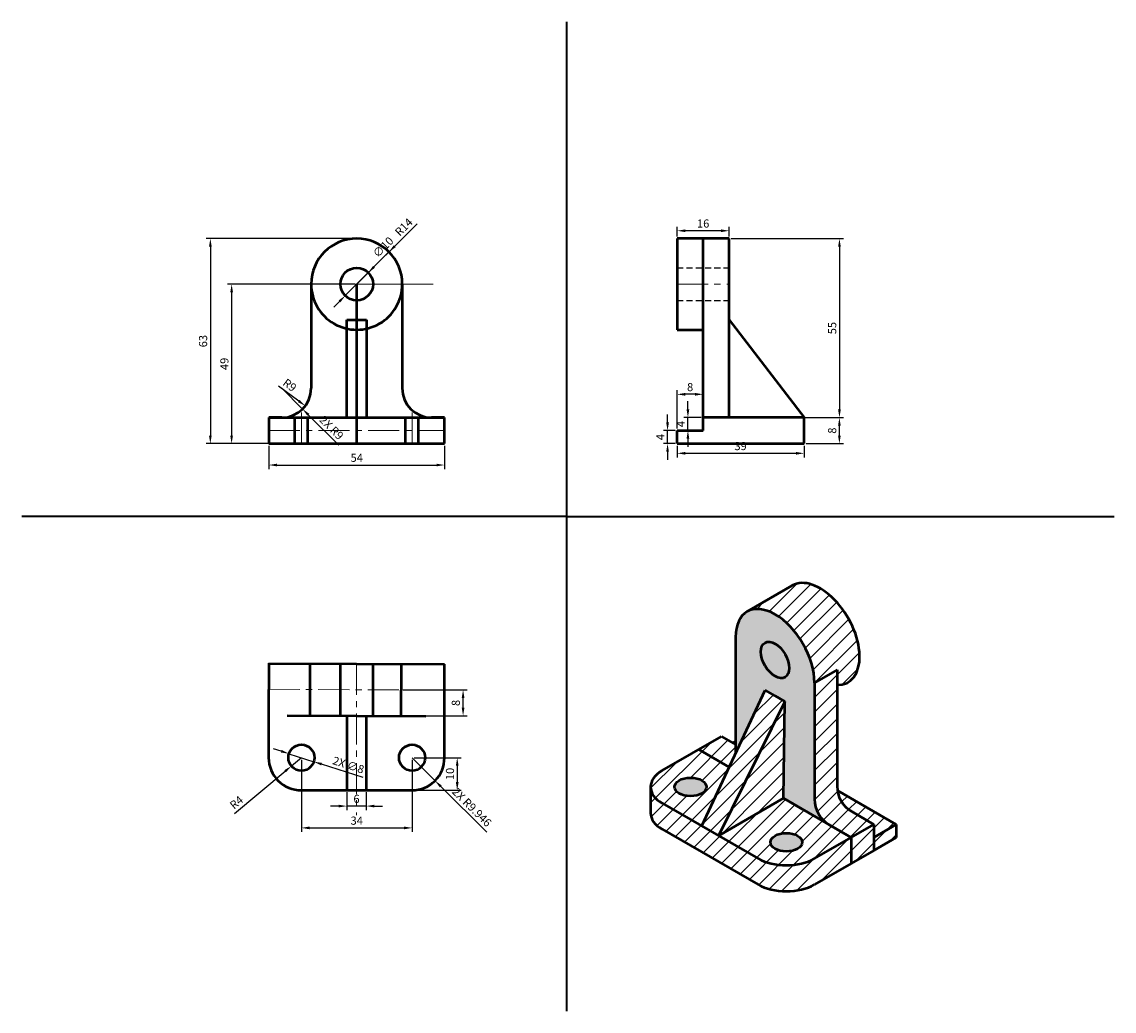
# Model space of a CAD drawing. Units: millimetres. Extents: x 2643 to 3341, y 1496 to 1804.
# Tile 2 of 2: x 3006 to 3341, y 1496 to 1800. Entities that reach past the tile are written whole.
import ezdxf

# ---------------------------------------------------------------- set-up
doc = ezdxf.new("R2010")
doc.units = ezdxf.units.MM
doc.linetypes.add('CENTER', pattern=[50.800000000000004, 31.75, -6.349999999999999, 6.349999999999999, -6.349999999999999])
doc.linetypes.add('HIDDEN', pattern=[9.524999999999999, 6.349999999999999, -3.174999999999999])
for name, color, linetype, lineweight in [('M-CNTR', 1, 'CENTER', 18), ('M-DIMS', 2, 'Continuous', 25), ('M-HATC', 252, 'Continuous', 18), ('M-HIDN', 4, 'HIDDEN', 25), ('M-OUTL', 7, 'Continuous', 50), ('M-TTLB', 8, 'Continuous', 35)]:
    doc.layers.add(name, color=color, linetype=linetype, lineweight=lineweight)
doc.styles.get("Standard").update_dxf_attribs({"font": 'arial.ttf'})
doc.dimstyles.new('ISO-25', dxfattribs={"dimtxt": 2.5, "dimasz": 2.5, "dimexe": 1.25, "dimexo": 0.625, "dimtad": 1, "dimtxsty": 'Standard', "dimcen": 2.5, "dimadec": 0, "dimazin": 0, "dimtfac": 1, "dimtmove": 0, "dimatfit": 3, "dimfxl": 1, "dimarcsym": 0})

# ---------------------------------------------------------------- blocks, each defined once
blk = doc.blocks.new('*D17')
at = {"layer": 'Defpoints', "color": 0, "transparency": 16777216}
for p in [(3081.566068859823, 1670.192632405238), (3135.566068859823, 1670.192632405237), (3135.566068859823, 1663.625483278832)]:
    blk.add_point(p, dxfattribs=at)
at = {"layer": 'M-DIMS', "color": 0, "lineweight": -2, "transparency": 16777216}
for p, q in [((3081.566068859823, 1669.567632405238), (3081.566068859823, 1662.375483278832)), ((3135.566068859823, 1669.567632405238), (3135.566068859823, 1662.375483278832)), ((3084.066068859823, 1663.625483278832), (3133.066068859823, 1663.625483278832))]:
    blk.add_line(p, q, dxfattribs=at)
at = {"layer": 'M-DIMS', "color": 0, "transparency": 16777216}
for points in [[(3084.066068859823, 1664.042149945499), (3084.066068859823, 1663.208816612165), (3081.566068859823, 1663.625483278832)], [(3133.066068859823, 1664.042149945499), (3133.066068859823, 1663.208816612165), (3135.566068859823, 1663.625483278832)]]:
    blk.add_solid(points, dxfattribs=at)
at = {"layer": 'M-DIMS', "color": 0, "transparency": 16777216, "insert": (3108.566068859823, 1665.521799786336), "char_height": 2.5, "attachment_point": 5}
blk.add_mtext('54', dxfattribs=at)
blk = doc.blocks.new('*D18')
at = {"layer": 'Defpoints', "color": 0, "transparency": 16777216}
for p in [(3085.566068859823, 1687.192632405238), (3092.76814055005, 1681.795395763327)]:
    blk.add_point(p, dxfattribs=at)
at = {"layer": 'M-DIMS', "color": 0, "lineweight": -2, "transparency": 16777216}
blk.add_line((3084.536577635948, 1687.964133716945), (3090.767565080541, 1683.294628163858), dxfattribs=at)
at = {"layer": 'M-DIMS', "color": 0, "transparency": 16777216}
blk.add_solid([(3091.017437147297, 1683.628057408776), (3090.517693013787, 1682.961198918941), (3092.76814055005, 1681.795395763327)], dxfattribs=at)
at = {"layer": 'M-DIMS', "color": 0, "transparency": 16777216, "insert": (3087.792059289652, 1687.900580802674), "char_height": 2.5, "attachment_point": 5, "rotation": 323.15208929564767}
blk.add_mtext('R9', dxfattribs=at)
blk = doc.blocks.new('*D19')
at = {"layer": 'Defpoints', "color": 0, "transparency": 16777216}
for p in [(3108.566068859825, 1719.192632405238), (3070.137380430236, 1670.192632405238), (3108.566068859825, 1670.192632405238)]:
    blk.add_point(p, dxfattribs=at)
at = {"layer": 'M-DIMS', "color": 0, "lineweight": -2, "transparency": 16777216}
for p, q in [((3107.941068859825, 1719.192632405238), (3068.887380430236, 1719.192632405238)), ((3070.137380430236, 1716.692632405238), (3070.137380430236, 1672.692632405238)), ((3107.941068859825, 1670.192632405238), (3068.887380430236, 1670.192632405238))]:
    blk.add_line(p, q, dxfattribs=at)
at = {"layer": 'M-DIMS', "color": 0, "transparency": 16777216}
for points in [[(3069.720713763569, 1716.692632405238), (3070.554047096902, 1716.692632405238), (3070.137380430236, 1719.192632405238)], [(3069.720713763569, 1672.692632405238), (3070.554047096902, 1672.692632405238), (3070.137380430236, 1670.192632405238)]]:
    blk.add_solid(points, dxfattribs=at)
at = {"layer": 'M-DIMS', "color": 0, "transparency": 16777216, "insert": (3068.235947960932, 1694.692632405236), "char_height": 2.5, "attachment_point": 5, "rotation": 90}
blk.add_mtext('49', dxfattribs=at)
blk = doc.blocks.new('*D20')
at = {"layer": 'Defpoints', "color": 0, "transparency": 16777216}
for p in [(3108.566068859825, 1733.192632405238), (3063.600548809042, 1670.192632405239), (3108.566068859825, 1670.192632405239)]:
    blk.add_point(p, dxfattribs=at)
at = {"layer": 'M-DIMS', "color": 0, "lineweight": -2, "transparency": 16777216}
for p, q in [((3107.941068859825, 1733.192632405238), (3062.350548809043, 1733.192632405238)), ((3063.600548809042, 1730.692632405238), (3063.600548809042, 1672.692632405239)), ((3107.941068859825, 1670.192632405239), (3062.350548809043, 1670.192632405239))]:
    blk.add_line(p, q, dxfattribs=at)
at = {"layer": 'M-DIMS', "color": 0, "transparency": 16777216}
for points in [[(3063.183882142376, 1730.692632405238), (3064.017215475709, 1730.692632405238), (3063.600548809042, 1733.192632405238)], [(3063.183882142376, 1672.692632405239), (3064.017215475709, 1672.692632405239), (3063.600548809042, 1670.192632405239)]]:
    blk.add_solid(points, dxfattribs=at)
at = {"layer": 'M-DIMS', "color": 0, "transparency": 16777216, "insert": (3061.698263679438, 1701.692632405237), "char_height": 2.5, "attachment_point": 5, "rotation": 90}
blk.add_mtext('63', dxfattribs=at)
blk = doc.blocks.new('*D21')
at = {"layer": 'Defpoints', "color": 0, "transparency": 16777216}
for p in [(3091.566068859822, 1573.72030741397), (3088.49388517497, 1571.158728329402)]:
    blk.add_point(p, dxfattribs=at)
at = {"layer": 'M-DIMS', "color": 0, "lineweight": -2, "transparency": 16777216}
for p, q in [((3091.566068859822, 1573.72030741397), (3088.49388517497, 1571.158728329402)), ((3071.01828682517, 1556.587618065424), (3086.573770371936, 1569.557741401545))]:
    blk.add_line(p, q, dxfattribs=at)
at = {"layer": 'M-DIMS', "color": 0, "transparency": 16777216}
blk.add_solid([(3086.306939217294, 1569.877760535384), (3086.840601526579, 1569.237722267706), (3088.49388517497, 1571.158728329402)], dxfattribs=at)
at = {"layer": 'M-DIMS', "color": 0, "transparency": 16777216, "insert": (3071.841787712557, 1559.715511328002), "char_height": 2.5, "attachment_point": 5, "rotation": 39.821262890870386}
blk.add_mtext('R4', dxfattribs=at)
blk = doc.blocks.new('*D22')
at = {"layer": 'Defpoints', "color": 0, "transparency": 16777216}
for p in [(3091.566068859821, 1573.720307413966), (3125.566068859823, 1573.72030741397), (3125.566068859823, 1552.148762047337)]:
    blk.add_point(p, dxfattribs=at)
at = {"layer": 'M-DIMS', "color": 0, "lineweight": -2, "transparency": 16777216}
for p, q in [((3091.566068859821, 1573.095307413966), (3091.566068859821, 1550.898762047337)), ((3125.566068859823, 1573.09530741397), (3125.566068859823, 1550.898762047337)), ((3094.066068859821, 1552.148762047337), (3123.066068859823, 1552.148762047337))]:
    blk.add_line(p, q, dxfattribs=at)
at = {"layer": 'M-DIMS', "color": 0, "transparency": 16777216}
for points in [[(3094.066068859821, 1552.565428714004), (3094.066068859821, 1551.73209538067), (3091.566068859821, 1552.148762047337)], [(3123.066068859823, 1552.565428714004), (3123.066068859823, 1551.73209538067), (3125.566068859823, 1552.148762047337)]]:
    blk.add_solid(points, dxfattribs=at)
at = {"layer": 'M-DIMS', "color": 0, "transparency": 16777216, "insert": (3108.566068859822, 1554.051047176942), "char_height": 2.5, "attachment_point": 5}
blk.add_mtext('34', dxfattribs=at)
blk = doc.blocks.new('*D23')
at = {"layer": 'Defpoints', "color": 0, "transparency": 16777216}
for p in [(3105.493192340093, 1563.72030741397), (3111.493192340093, 1563.720307413971), (3105.493192340093, 1558.848600236895)]:
    blk.add_point(p, dxfattribs=at)
at = {"layer": 'M-DIMS', "color": 0, "lineweight": -2, "transparency": 16777216}
for p, q in [((3105.493192340093, 1563.095307413971), (3105.493192340093, 1557.598600236896)), ((3111.493192340093, 1563.095307413971), (3111.493192340093, 1557.598600236896)), ((3102.993192340093, 1558.848600236895), (3100.493192340093, 1558.848600236895)), ((3111.493192340093, 1558.848600236895), (3105.493192340093, 1558.848600236895)), ((3113.993192340093, 1558.848600236895), (3116.493192340093, 1558.848600236895))]:
    blk.add_line(p, q, dxfattribs=at)
at = {"layer": 'M-DIMS', "color": 0, "transparency": 16777216}
for points in [[(3102.993192340093, 1559.265266903562), (3102.993192340093, 1558.431933570229), (3105.493192340093, 1558.848600236895)], [(3113.993192340093, 1559.265266903562), (3113.993192340093, 1558.431933570229), (3111.493192340093, 1558.848600236895)]]:
    blk.add_solid(points, dxfattribs=at)
at = {"layer": 'M-DIMS', "color": 0, "transparency": 16777216, "insert": (3108.493192340093, 1560.7500327062), "char_height": 2.5, "attachment_point": 5}
blk.add_mtext('6', dxfattribs=at)
blk = doc.blocks.new('*D24')
at = {"layer": 'Defpoints', "color": 0, "transparency": 16777216}
for p in [(3125.566068859825, 1573.720307413971), (3125.593251720514, 1563.720344158577), (3139.428818305797, 1563.720344158577)]:
    blk.add_point(p, dxfattribs=at)
at = {"layer": 'M-DIMS', "color": 0, "lineweight": -2, "transparency": 16777216}
for p, q in [((3126.191068859825, 1573.720307413971), (3140.678818305797, 1573.720307413971)), ((3139.428818305797, 1571.220307413971), (3139.428818305797, 1566.220344158577)), ((3126.218251720513, 1563.720344158577), (3140.678818305797, 1563.720344158577))]:
    blk.add_line(p, q, dxfattribs=at)
at = {"layer": 'M-DIMS', "color": 0, "transparency": 16777216}
for points in [[(3139.012151639131, 1571.220307413971), (3139.845484972464, 1571.220307413971), (3139.428818305797, 1573.720307413971)], [(3139.012151639131, 1566.220344158577), (3139.845484972464, 1566.220344158577), (3139.428818305797, 1563.720344158577)]]:
    blk.add_solid(points, dxfattribs=at)
at = {"layer": 'M-DIMS', "color": 0, "transparency": 16777216, "insert": (3137.527385836492, 1568.720325786273), "char_height": 2.5, "attachment_point": 5, "rotation": 90}
blk.add_mtext('10', dxfattribs=at)
blk = doc.blocks.new('*D25')
at = {"layer": 'Defpoints', "color": 0, "transparency": 16777216}
for p in [(3122.144030181128, 1594.535232754655), (3141.230326541379, 1594.535232754655), (3122.315422410063, 1586.534369106776)]:
    blk.add_point(p, dxfattribs=at)
at = {"layer": 'M-DIMS', "color": 0, "lineweight": -2, "transparency": 16777216}
for p, q in [((3122.769030181129, 1594.535232754655), (3142.480326541379, 1594.535232754655)), ((3141.230326541379, 1589.034369106776), (3141.230326541379, 1592.035232754655)), ((3122.940422410063, 1586.534369106776), (3142.480326541379, 1586.534369106776))]:
    blk.add_line(p, q, dxfattribs=at)
at = {"layer": 'M-DIMS', "color": 0, "transparency": 16777216}
for points in [[(3140.813659874712, 1592.035232754655), (3141.646993208045, 1592.035232754655), (3141.230326541379, 1594.535232754655)], [(3140.813659874712, 1589.034369106776), (3141.646993208045, 1589.034369106776), (3141.230326541379, 1586.534369106776)]]:
    blk.add_solid(points, dxfattribs=at)
at = {"layer": 'M-DIMS', "color": 0, "transparency": 16777216, "insert": (3139.328894072074, 1590.534800930714), "char_height": 2.5, "attachment_point": 5, "rotation": 90}
blk.add_mtext('8', dxfattribs=at)
blk = doc.blocks.new('*D26')
at = {"layer": 'Defpoints', "color": 0, "transparency": 16777216}
for p in [(3206.974275947713, 1735.593289619921), (3206.974275947713, 1733.192632405237), (3222.974275947713, 1733.192632405237)]:
    blk.add_point(p, dxfattribs=at)
at = {"layer": 'M-DIMS', "color": 0, "lineweight": -2, "transparency": 16777216}
for p, q in [((3206.974275947713, 1733.817632405237), (3206.974275947713, 1736.843289619922)), ((3220.474275947713, 1735.593289619921), (3209.474275947713, 1735.593289619921)), ((3222.974275947713, 1733.817632405237), (3222.974275947713, 1736.843289619922))]:
    blk.add_line(p, q, dxfattribs=at)
at = {"layer": 'M-DIMS', "color": 0, "transparency": 16777216}
for points in [[(3209.474275947713, 1736.009956286588), (3209.474275947713, 1735.176622953255), (3206.974275947713, 1735.593289619921)], [(3220.474275947713, 1736.009956286588), (3220.474275947713, 1735.176622953255), (3222.974275947713, 1735.593289619921)]]:
    blk.add_solid(points, dxfattribs=at)
at = {"layer": 'M-DIMS', "color": 0, "transparency": 16777216, "insert": (3214.974275947713, 1737.494722089225), "char_height": 2.5, "attachment_point": 5}
blk.add_mtext('16', dxfattribs=at)
blk = doc.blocks.new('*D27')
at = {"layer": 'Defpoints', "color": 0, "transparency": 16777216}
for p in [(3206.974275947713, 1685.342880000957), (3206.974275947713, 1674.192632405237), (3214.974275947713, 1674.192632405237)]:
    blk.add_point(p, dxfattribs=at)
at = {"layer": 'M-DIMS', "color": 0, "lineweight": -2, "transparency": 16777216}
for p, q in [((3206.974275947713, 1674.817632405237), (3206.974275947713, 1686.592880000956)), ((3212.474275947713, 1685.342880000957), (3209.474275947713, 1685.342880000957)), ((3214.974275947713, 1674.817632405237), (3214.974275947713, 1686.592880000956))]:
    blk.add_line(p, q, dxfattribs=at)
at = {"layer": 'M-DIMS', "color": 0, "transparency": 16777216}
for points in [[(3209.474275947713, 1685.759546667623), (3209.474275947713, 1684.92621333429), (3206.974275947713, 1685.342880000957)], [(3212.474275947713, 1685.759546667623), (3212.474275947713, 1684.92621333429), (3214.974275947713, 1685.342880000957)]]:
    blk.add_solid(points, dxfattribs=at)
at = {"layer": 'M-DIMS', "color": 0, "transparency": 16777216, "insert": (3210.974275947713, 1687.244312470261), "char_height": 2.5, "attachment_point": 5}
blk.add_mtext('8', dxfattribs=at)
blk = doc.blocks.new('*D28')
at = {"layer": 'Defpoints', "color": 0, "transparency": 16777216}
for p in [(3204.041964908853, 1674.192632405238), (3206.974275947715, 1674.192632405238), (3206.974275947715, 1670.192632405238)]:
    blk.add_point(p, dxfattribs=at)
at = {"layer": 'M-DIMS', "color": 0, "lineweight": -2, "transparency": 16777216}
for p, q in [((3204.041964908853, 1676.692632405238), (3204.041964908853, 1679.192632405239)), ((3206.349275947715, 1674.192632405238), (3202.791964908853, 1674.192632405238)), ((3204.041964908853, 1670.192632405238), (3204.041964908853, 1674.192632405238)), ((3206.349275947715, 1670.192632405238), (3202.791964908853, 1670.192632405238)), ((3204.041964908853, 1667.692632405238), (3204.041964908853, 1665.192632405238))]:
    blk.add_line(p, q, dxfattribs=at)
at = {"layer": 'M-DIMS', "color": 0, "transparency": 16777216}
for points in [[(3203.625298242187, 1676.692632405238), (3204.458631575519, 1676.692632405238), (3204.041964908853, 1674.192632405238)], [(3203.625298242187, 1667.692632405238), (3204.458631575519, 1667.692632405238), (3204.041964908853, 1670.192632405238)]]:
    blk.add_solid(points, dxfattribs=at)
at = {"layer": 'M-DIMS', "color": 0, "transparency": 16777216, "insert": (3202.166964908852, 1672.192632405237), "char_height": 2.5, "attachment_point": 5, "rotation": 90}
blk.add_mtext('4', dxfattribs=at)
blk = doc.blocks.new('*D29')
at = {"layer": 'Defpoints', "color": 0, "transparency": 16777216}
for p in [(3210.288262918699, 1678.192632405238), (3214.974275947715, 1678.192632405238), (3214.974275947715, 1674.192632405238)]:
    blk.add_point(p, dxfattribs=at)
at = {"layer": 'M-DIMS', "color": 0, "lineweight": -2, "transparency": 16777216}
for p, q in [((3210.288262918699, 1680.692632405239), (3210.288262918699, 1683.192632405238)), ((3214.349275947715, 1678.192632405238), (3209.038262918699, 1678.192632405238)), ((3210.288262918699, 1674.192632405238), (3210.288262918699, 1678.192632405238)), ((3214.349275947715, 1674.192632405238), (3209.038262918699, 1674.192632405238)), ((3210.288262918699, 1671.692632405239), (3210.288262918699, 1669.192632405238))]:
    blk.add_line(p, q, dxfattribs=at)
at = {"layer": 'M-DIMS', "color": 0, "transparency": 16777216}
for points in [[(3209.871596252033, 1680.692632405239), (3210.704929585366, 1680.692632405239), (3210.288262918699, 1678.192632405238)], [(3209.871596252033, 1671.692632405239), (3210.704929585366, 1671.692632405239), (3210.288262918699, 1674.192632405238)]]:
    blk.add_solid(points, dxfattribs=at)
at = {"layer": 'M-DIMS', "color": 0, "transparency": 16777216, "insert": (3208.413262918699, 1676.192632405237), "char_height": 2.5, "attachment_point": 5, "rotation": 90}
blk.add_mtext('4', dxfattribs=at)
blk = doc.blocks.new('*D30')
at = {"layer": 'Defpoints', "color": 0, "transparency": 16777216}
for p in [(3206.974275947713, 1670.192632405237), (3245.974275947713, 1670.192632405237), (3245.974275947713, 1667.224246976519)]:
    blk.add_point(p, dxfattribs=at)
at = {"layer": 'M-DIMS', "color": 0, "lineweight": -2, "transparency": 16777216}
for p, q in [((3206.974275947713, 1669.567632405238), (3206.974275947713, 1665.974246976519)), ((3245.974275947713, 1669.567632405238), (3245.974275947713, 1665.974246976519)), ((3209.474275947713, 1667.224246976519), (3243.474275947713, 1667.224246976519))]:
    blk.add_line(p, q, dxfattribs=at)
at = {"layer": 'M-DIMS', "color": 0, "transparency": 16777216}
for points in [[(3209.474275947713, 1667.640913643186), (3209.474275947713, 1666.807580309852), (3206.974275947713, 1667.224246976519)], [(3243.474275947713, 1667.640913643186), (3243.474275947713, 1666.807580309852), (3245.974275947713, 1667.224246976519)]]:
    blk.add_solid(points, dxfattribs=at)
at = {"layer": 'M-DIMS', "color": 0, "transparency": 16777216, "insert": (3226.474275947713, 1669.126532106123), "char_height": 2.5, "attachment_point": 5}
blk.add_mtext('39', dxfattribs=at)
blk = doc.blocks.new('*D31')
at = {"layer": 'Defpoints', "color": 0, "transparency": 16777216}
for p in [(3245.974275947715, 1678.192632405238), (3256.821093267697, 1678.192632405238), (3245.974275947715, 1670.192632405238)]:
    blk.add_point(p, dxfattribs=at)
at = {"layer": 'M-DIMS', "color": 0, "lineweight": -2, "transparency": 16777216}
for p, q in [((3246.599275947715, 1678.192632405238), (3258.071093267697, 1678.192632405238)), ((3256.821093267697, 1672.692632405238), (3256.821093267697, 1675.692632405239)), ((3246.599275947715, 1670.192632405238), (3258.071093267697, 1670.192632405238))]:
    blk.add_line(p, q, dxfattribs=at)
at = {"layer": 'M-DIMS', "color": 0, "transparency": 16777216}
for points in [[(3256.40442660103, 1675.692632405239), (3257.237759934363, 1675.692632405239), (3256.821093267697, 1678.192632405238)], [(3256.40442660103, 1672.692632405238), (3257.237759934363, 1672.692632405238), (3256.821093267697, 1670.192632405238)]]:
    blk.add_solid(points, dxfattribs=at)
at = {"layer": 'M-DIMS', "color": 0, "transparency": 16777216, "insert": (3254.919660798392, 1674.192632405237), "char_height": 2.5, "attachment_point": 5, "rotation": 90}
blk.add_mtext('8', dxfattribs=at)
blk = doc.blocks.new('*D32')
at = {"layer": 'Defpoints', "color": 0, "transparency": 16777216}
for p in [(3222.974275947715, 1733.192632405238), (3222.974275947715, 1678.192632405238), (3256.830360983441, 1678.192632405238)]:
    blk.add_point(p, dxfattribs=at)
at = {"layer": 'M-DIMS', "color": 0, "lineweight": -2, "transparency": 16777216}
for p, q in [((3223.599275947715, 1733.192632405238), (3258.080360983441, 1733.192632405238)), ((3256.830360983441, 1730.692632405238), (3256.830360983441, 1680.692632405239)), ((3223.599275947715, 1678.192632405238), (3258.080360983441, 1678.192632405238))]:
    blk.add_line(p, q, dxfattribs=at)
at = {"layer": 'M-DIMS', "color": 0, "transparency": 16777216}
for points in [[(3256.413694316775, 1730.692632405238), (3257.247027650108, 1730.692632405238), (3256.830360983441, 1733.192632405238)], [(3256.413694316775, 1680.692632405239), (3257.247027650108, 1680.692632405239), (3256.830360983441, 1678.192632405238)]]:
    blk.add_solid(points, dxfattribs=at)
at = {"layer": 'M-DIMS', "color": 0, "transparency": 16777216, "insert": (3254.934044475938, 1705.692632405237), "char_height": 2.5, "attachment_point": 5, "rotation": 90}
blk.add_mtext('55', dxfattribs=at)
blk = doc.blocks.new('*D40')
at = {"layer": 'Defpoints', "color": 0, "transparency": 16777216}
for p in [(3085.566069, 1687.192632), (3091.930179000001, 1680.828820999999)]:
    blk.add_point(p, dxfattribs=at)
at = {"layer": 'M-DIMS', "color": 0, "lineweight": -2, "transparency": 16777216}
for p, q in [((3085.566069, 1687.192632), (3091.930179000001, 1680.828820999999)), ((3103.032643309519, 1669.726878308875), (3093.697987480261, 1679.061095575302))]:
    blk.add_line(p, q, dxfattribs=at)
at = {"layer": 'M-DIMS', "color": 0, "transparency": 16777216}
blk.add_solid([(3093.992608384378, 1679.355730322012), (3093.403366576145, 1678.766460828592), (3091.930179000001, 1680.828820999999)], dxfattribs=at)
at = {"layer": 'M-DIMS', "color": 0, "transparency": 16777216, "insert": (3100.593703842754, 1674.854671607291), "char_height": 2.5, "attachment_point": 5, "rotation": 315.0013459730079}
blk.add_mtext('2X R9', dxfattribs=at)
blk = doc.blocks.new('*D41')
at = {"layer": 'Defpoints', "color": 0, "transparency": 16777216}
for p in [(3112.099884, 1722.729884), (3105.032254000001, 1715.65538)]:
    blk.add_point(p, dxfattribs=at)
at = {"layer": 'M-DIMS', "color": 0, "lineweight": -2, "transparency": 16777216}
for p, q in [((3120.964552908202, 1731.603174714109), (3113.866791494144, 1724.498509994138)), ((3105.032254000001, 1715.65538), (3112.099884, 1722.729884)), ((3103.265346505857, 1713.886754005862), (3101.498439011714, 1712.118128011724))]:
    blk.add_line(p, q, dxfattribs=at)
at = {"layer": 'M-DIMS', "color": 0, "transparency": 16777216}
for points in [[(3113.572020495121, 1724.792994576495), (3114.161562493166, 1724.20402541178), (3112.099884, 1722.729884)], [(3102.970575506834, 1714.181238588219), (3103.56011750488, 1713.592269423504), (3105.032254000001, 1715.65538)]]:
    blk.add_solid(points, dxfattribs=at)
at = {"layer": 'M-DIMS', "color": 0, "transparency": 16777216, "insert": (3116.904493172512, 1730.328433020517), "char_height": 2.5, "attachment_point": 5, "rotation": 45.02784948561538}
blk.add_mtext('∅10', dxfattribs=at)
blk = doc.blocks.new('*D42')
at = {"layer": 'Defpoints', "color": 0, "transparency": 16777216}
for p in [(3118.468845000001, 1729.088845000001), (3108.566069, 1719.192631999999)]:
    blk.add_point(p, dxfattribs=at)
at = {"layer": 'M-DIMS', "color": 0, "lineweight": -2, "transparency": 16777216}
for p, q in [((3127.107960297154, 1737.722234780015), (3120.237197837983, 1730.856025873709)), ((3108.566069, 1719.192631999999), (3118.468845000001, 1729.088845000001))]:
    blk.add_line(p, q, dxfattribs=at)
at = {"layer": 'M-DIMS', "color": 0, "transparency": 16777216}
blk.add_solid([(3119.942667692365, 1731.150751346706), (3120.531727983601, 1730.561300400712), (3118.468845000001, 1729.088845000001)], dxfattribs=at)
at = {"layer": 'M-DIMS', "color": 0, "transparency": 16777216, "insert": (3123.227753499339, 1736.502604122431), "char_height": 2.5, "attachment_point": 5, "rotation": 44.98100750562735}
blk.add_mtext('R14', dxfattribs=at)
blk = doc.blocks.new('*D43')
at = {"layer": 'Defpoints', "color": 0, "transparency": 16777216}
for p in [(3087.758719, 1574.946716), (3095.373418999999, 1572.493898)]:
    blk.add_point(p, dxfattribs=at)
at = {"layer": 'M-DIMS', "color": 0, "lineweight": -2, "transparency": 16777216}
for p, q in [((3085.37912473376, 1575.713221791289), (3082.999530467521, 1576.479727582579)), ((3087.758719, 1574.946716), (3095.373418999999, 1572.493898)), ((3110.503158533163, 1567.620364247881), (3097.753013266239, 1571.727392208711))]:
    blk.add_line(p, q, dxfattribs=at)
at = {"layer": 'M-DIMS', "color": 0, "transparency": 16777216}
for points in [[(3085.506875698975, 1576.109820835662), (3085.251373768545, 1575.316622746916), (3087.758719, 1574.946716)], [(3097.880764231453, 1572.123991253084), (3097.625262301024, 1571.330793164337), (3095.373418999999, 1572.493898)]]:
    blk.add_solid(points, dxfattribs=at)
at = {"layer": 'M-DIMS', "color": 0, "transparency": 16777216, "insert": (3105.922303697712, 1571.1670311797), "char_height": 2.5, "attachment_point": 5, "rotation": 342.14541089494566}
blk.add_mtext('2X ∅8', dxfattribs=at)
blk = doc.blocks.new('*D44')
at = {"layer": 'Defpoints', "color": 0, "transparency": 16777216}
for p in [(3125.566216000002, 1573.666236), (3132.617793, 1566.652196)]:
    blk.add_point(p, dxfattribs=at)
at = {"layer": 'M-DIMS', "color": 0, "lineweight": -2, "transparency": 16777216}
for p, q in [((3125.566216000002, 1573.666236), (3132.617793, 1566.652196)), ((3148.564052339653, 1550.790821890534), (3134.390271291905, 1564.889152975928))]:
    blk.add_line(p, q, dxfattribs=at)
at = {"layer": 'M-DIMS', "color": 0, "transparency": 16777216}
blk.add_solid([(3134.684111795916, 1565.184566024579), (3134.096430787893, 1564.593739927278), (3132.617793, 1566.652196)], dxfattribs=at)
at = {"layer": 'M-DIMS', "color": 0, "transparency": 16777216, "insert": (3143.704323862031, 1558.306565031341), "char_height": 2.5, "attachment_point": 5, "rotation": 315.15290524189516}
blk.add_mtext('2X R9.946', dxfattribs=at)

msp = doc.modelspace()

# ---------------------------------------------------------------- hatches: boundary and pattern name
at = {"layer": 'M-HATC'}
h = msp.add_hatch(dxfattribs=at)
h.set_pattern_fill('ANSI31', color=256)
h.set_pattern_definition([(45, (-305.4882711523164, 13.1998327818701), (-2.245064030267288, 2.245064030267288), [])])
edge = h.paths.add_edge_path()
edge.add_ellipse((3250.910199354826, 1611.738493132284), major_axis=(8.573214099741039, -14.84924240491754), ratio=0.577350269189623, start_angle=348.3683023236149, end_angle=540)
edge.add_line((3242.336985255085, 1626.587735537202), (3228.480578794533, 1618.587735537202))
edge.add_ellipse((3237.053792894275, 1603.738493132284), major_axis=(8.573214099741039, -14.84924240491754), ratio=0.577350269189623, start_angle=390.0000000000002, end_angle=540.0000000000002, ccw=False)
edge.add_line((3249.178148547257, 1596.738493132284), (3256.106351777532, 1600.738493132285))
edge.add_line((3256.106351777532, 1600.738493132285), (3256.106351777532, 1596.089382491611))
h.paths.add_polyline_path([(3256.106351777532, 1600.738493132285), (3249.178148547257, 1596.738493132284), (3249.178148547257, 1560.934645554991, 0.2679491924311224), (3253.678148547257, 1553.140416920931), (3260.436478796454, 1549.238493132284), (3267.364682026729, 1553.238493132284), (3260.606351777532, 1557.140416920931, -0.2679491924311224), (3256.106351777532, 1564.934645554991)])
h.paths.add_polyline_path([(3274.292885257005, 1553.238493132284), (3256.193048909, 1563.688438520093, 0.2310558315879979), (3260.606351777532, 1557.140416920931), (3267.364682026729, 1553.238493132284), (3267.364682026729, 1549.238493132284)])
h.paths.add_polyline_path([(3274.292885257005, 1553.238493132284), (3267.364682026729, 1549.238493132284), (3267.364682026729, 1545.238493132284), (3274.292885257005, 1549.238493132284)])
h.paths.add_polyline_path([(3267.364682026729, 1549.238493132284), (3267.364682026729, 1553.238493132284), (3260.436478796454, 1549.238493132284), (3260.436478796454, 1541.238493132284), (3267.364682026729, 1545.238493132284)])
edge = h.paths.add_edge_path()
edge.add_line((3260.436478796454, 1541.238493132284), (3260.436478796454, 1549.238493132284))
edge.add_line((3260.436478796454, 1549.238493132284), (3249.178148547257, 1542.738493132284))
edge.add_ellipse((3240.517894509412, 1547.738493132284), major_axis=(-12.24744871391593, 0), ratio=0.5773502691896287, start_angle=29.999999999999886, end_angle=150.0000000000001, ccw=False)
edge.add_line((3231.857640471568, 1542.738493132284), (3202.412776742896, 1559.738493132284))
edge.add_ellipse((3211.073030780742, 1564.738493132284), major_axis=(-12.24744871391593, 0), ratio=0.5773502691896287, start_angle=360, end_angle=389.9999999999999, ccw=False)
edge.add_line((3198.825582066825, 1563.994951168402), (3198.825582066825, 1556.738493132284))
edge.add_ellipse((3211.073030780742, 1556.738493132284), major_axis=(-12.24744871391593, 0), ratio=0.5773502691896287, start_angle=360, end_angle=389.9999999999999)
edge.add_line((3202.412776742896, 1551.738493132284), (3231.857640471568, 1534.738493132284))
edge.add_ellipse((3240.517894509412, 1539.738493132284), major_axis=(-12.24744871391593, 0), ratio=0.5773502691896287, start_angle=29.9999999999999, end_angle=150.0000000000001)
edge.add_line((3249.178148547257, 1534.738493132284), (3260.436478796454, 1541.238493132284))
edge = h.paths.add_edge_path(flags=17)
edge.add_line((3260.436478796454, 1549.238493132284), (3253.678148547257, 1553.140416920931))
edge.add_line((3253.678148547257, 1553.140416920931), (3239.651869105628, 1561.238493132284))
edge.add_line((3239.651869105628, 1561.238493132284), (3219.733284818586, 1549.738493132284))
edge.add_line((3219.733284818586, 1549.738493132284), (3231.857640471568, 1542.738493132284))
edge.add_ellipse((3240.517894509412, 1547.738493132284), major_axis=(-12.24744871391593, 0), ratio=0.5773502691896287, start_angle=29.9999999999999, end_angle=150.0000000000001)
edge.add_line((3249.178148547257, 1542.738493132284), (3260.436478796454, 1549.238493132284))
edge = h.paths.add_edge_path(flags=16)
edge.add_ellipse((3240.517894509412, 1547.738493132284), major_axis=(-4.898979485566355, 0), ratio=0.5773502691896306, start_angle=0, end_angle=360)
h.paths.add_polyline_path([(3239.651869105628, 1561.238493132284), (3240.084881807521, 1590.988493132284), (3219.733284818586, 1549.738493132284)], flags=17)
h.paths.add_polyline_path([(3240.084881807521, 1590.988493132284), (3237.053792894275, 1592.738493132284), (3234.022703981029, 1594.488493132284), (3214.537132395879, 1552.738493132284), (3219.733284818586, 1549.738493132284)])
edge = h.paths.add_edge_path()
edge.add_line((3222.993135159246, 1570.856417660586), (3213.671106992094, 1576.238493132284))
edge.add_line((3213.671106992094, 1576.238493132284), (3202.412776742896, 1569.738493132284))
edge.add_ellipse((3211.073030780742, 1564.738493132284), major_axis=(-12.24744871391593, 0), ratio=0.5773502691896287, start_angle=330.0000000000001, end_angle=360)
edge.add_ellipse((3211.073030780742, 1564.738493132284), major_axis=(-12.24744871391593, 0), ratio=0.5773502691896287, start_angle=360, end_angle=389.9999999999999)
edge.add_line((3202.4127767429, 1559.738493132283), (3214.537132395879, 1552.738493132284))
edge.add_line((3214.537132395879, 1552.738493132284), (3222.993135159246, 1570.856417660586))
edge = h.paths.add_edge_path(flags=16)
edge.add_ellipse((3211.073030780742, 1564.738493132284), major_axis=(-4.898979485566355, 0), ratio=0.5773502691896306, start_angle=0, end_angle=360)
h.paths.add_polyline_path([(3224.929437241293, 1577.738493132284), (3220.59931022237, 1580.238493132284), (3213.671106992094, 1576.238493132284), (3222.993135159246, 1570.856417660586), (3224.929437241293, 1575.005159798951)])
h = msp.add_hatch(color=256, dxfattribs=at)
h.dxf.hatch_style = 1
edge = h.paths.add_edge_path()
edge.add_ellipse((3237.053792894275, 1603.738493132284), major_axis=(8.573214099741039, -14.84924240491754), ratio=0.577350269189623, start_angle=30.00000000000186, end_angle=210.0000000000002)
edge.add_line((3224.929437241293, 1610.738493132284), (3224.929437241293, 1575.005159798952))
edge.add_line((3224.929437241293, 1575.005159798952), (3234.022703981029, 1594.488493132284))
edge.add_line((3234.022703981029, 1594.488493132284), (3237.053792894274, 1592.738493132284))
edge.add_line((3237.053792894274, 1592.738493132284), (3240.084881807521, 1590.988493132284))
edge.add_line((3240.084881807521, 1590.988493132284), (3239.651869105629, 1561.238493132284))
edge.add_line((3239.651869105629, 1561.238493132284), (3253.678148547257, 1553.140416920931))
edge.add_arc((3258.178148547257, 1560.934645554991), 8.999999999999893, 180, 239.9999999999999, ccw=False)
edge.add_line((3249.178148547257, 1560.934645554991), (3249.178148547257, 1596.738493132285))
edge = h.paths.add_edge_path(flags=16)
edge.add_ellipse((3237.053792894275, 1603.738493132284), major_axis=(3.061862178479193, -5.303300858898984), ratio=0.5773502691896079, start_angle=0, end_angle=360)
edge = h.paths.add_edge_path()
edge.add_ellipse((3211.073030780742, 1564.738493132284), major_axis=(-4.898979485566355, 0), ratio=0.5773502691896306, start_angle=0, end_angle=360)
edge = h.paths.add_edge_path()
edge.add_ellipse((3240.517894509412, 1547.738493132284), major_axis=(-4.898979485566355, 0), ratio=0.5773502691896306, start_angle=0, end_angle=360)
h = msp.add_hatch(color=256, dxfattribs=at)
h.dxf.hatch_style = 1
edge = h.paths.add_edge_path()
edge.add_ellipse((3237.053792894275, 1603.738493132284), major_axis=(3.061862178479193, -5.303300858898984), ratio=0.5773502691896079, start_angle=0, end_angle=360)

# ---------------------------------------------------------------- linework, layer by layer
at = {"layer": 'M-CNTR'}
for q in [(3077.880164466212, 1719.192632405238), (3132.062269911445, 1719.192632405238)]:
    msp.add_line((3108.566068859823, 1719.192632405238), q, dxfattribs=at)
at = {"layer": 'M-CNTR', "ltscale": 0.3}
for p, q in [((3206.974275947713, 1719.192632405238), (3222.974275947713, 1719.192632405238)), ((3091.566068859823, 1670.192632405237), (3091.566068859823, 1680.484428472738)), ((3125.566068859823, 1670.192632405237), (3125.566068859823, 1680.484428472738)), ((3081.566068859823, 1674.192632405237), (3135.566068859823, 1674.192632405237)), ((3108.493192340092, 1602.552277963965), (3108.493192340092, 1556.097798737711)), ((3081.529630599958, 1594.720224429366), (3135.529630599958, 1594.474263623908))]:
    msp.add_line(p, q, dxfattribs=at)
at = {"layer": 'M-HIDN', "ltscale": 0.3}
for p, q in [((3206.974275947713, 1724.192632405237), (3222.974275947713, 1724.192632405237)), ((3206.974275947713, 1714.192632405238), (3222.974275947713, 1714.192632405238))]:
    msp.add_line(p, q, dxfattribs=at)
at = {"layer": 'M-OUTL'}
for p, q in [((3222.974275947713, 1733.192632405237), (3206.974275947713, 1733.192632405237)), ((3206.974275947713, 1733.192632405237), (3206.974275947713, 1705.192632405237)), ((3214.974275947713, 1678.192632405238), (3214.974275947713, 1733.192632405237)), ((3222.974275947713, 1678.192632405238), (3222.974275947713, 1733.192632405237)), ((3094.566068859823, 1719.192632405238), (3094.566068859823, 1687.192632405238)), ((3108.566068859823, 1670.192632405237), (3108.566068859823, 1719.192632405238)), ((3122.566068859823, 1719.192632405237), (3122.566068859823, 1687.192632405237)), ((3105.566068859823, 1678.192632405238), (3105.566068859823, 1708.192632405237)), ((3105.566068859823, 1708.192632405237), (3111.566068859823, 1708.192632405237)), ((3111.566068859823, 1708.192632405237), (3111.566068859823, 1678.192632405238)), ((3222.974275947713, 1708.192632405238), (3245.974275947713, 1678.192632405238)), ((3206.974275947713, 1705.192632405237), (3214.974275947713, 1705.192632405237)), ((3085.566068859823, 1678.192632405238), (3081.566068859823, 1678.192632405238)), ((3081.566068859823, 1678.192632405238), (3081.566068859823, 1670.192632405237)), ((3081.566068859823, 1678.192632405238), (3135.566068859823, 1678.192632405238)), ((3089.566068859823, 1670.192632405237), (3089.566068859822, 1678.192632405238)), ((3093.566068859823, 1670.192632405237), (3093.566068859824, 1678.192632405238)), ((3123.566068859823, 1670.192632405237), (3123.566068859823, 1678.192632405238)), ((3127.566068859823, 1670.192632405237), (3127.566068859823, 1678.192632405238)), ((3135.566068859823, 1678.192632405238), (3131.566068859823, 1678.192632405238)), ((3135.566068859823, 1670.192632405237), (3135.566068859823, 1678.192632405238)), ((3214.974275947713, 1674.192632405237), (3214.974275947713, 1678.192632405238)), ((3245.974275947713, 1678.192632405238), (3214.974275947713, 1678.192632405238)), ((3245.974275947713, 1670.192632405237), (3245.974275947713, 1678.192632405238)), ((3206.974275947713, 1670.192632405237), (3206.974275947713, 1674.192632405237)), ((3206.974275947713, 1674.192632405237), (3214.974275947713, 1674.192632405237)), ((3081.566068859823, 1670.192632405237), (3135.566068859823, 1670.192632405237)), ((3206.974275947713, 1670.192632405237), (3245.974275947713, 1670.192632405237)), ((3228.480578794533, 1618.587735537202), (3242.336985255085, 1626.587735537202)), ((3224.929437241293, 1610.738493132284), (3224.929437241293, 1575.005159798951)), ((3081.566068859823, 1602.720141444761), (3081.493192340094, 1586.72030741397)), ((3081.565862917386, 1602.674927364588), (3135.512144286759, 1602.429211238347)), ((3094.181049330208, 1602.662682356663), (3094.108172810479, 1586.662848325871)), ((3103.493192340092, 1602.552277963965), (3103.493192340092, 1586.597327011246)), ((3113.493192340092, 1602.552277963965), (3113.493192340092, 1586.597327011246)), ((3122.180468440991, 1602.535149770055), (3122.107591921261, 1586.535315739263)), ((3135.512144286759, 1573.66623585732), (3135.512144286759, 1602.429211238347)), ((3256.106351777532, 1600.738493132285), (3249.178148547257, 1596.738493132285)), ((3256.106351777532, 1600.738493132285), (3256.106351777532, 1564.934645554991)), ((3214.537132395879, 1552.738493132284), (3234.022703981029, 1594.488493132284)), ((3237.053792894274, 1592.738493132284), (3234.022703981029, 1594.488493132284)), ((3249.178148547257, 1596.738493132285), (3249.178148547257, 1560.934645554991)), ((3240.084881807521, 1590.988493132284), (3219.733284818588, 1549.738493132284)), ((3237.053792894274, 1592.738493132284), (3240.084881807521, 1590.988493132284)), ((3239.651869105629, 1561.238493132284), (3240.084881807521, 1590.988493132284)), ((3081.493192340094, 1586.72030741397), (3081.493192340094, 1573.719776305331)), ((3087.230272094596, 1586.694175992538), (3129.756113831807, 1586.500478024271)), ((3105.493192963201, 1586.597327008407), (3105.493192340093, 1563.720307413971)), ((3111.493192963201, 1586.597327008407), (3111.493192340093, 1563.720307413971)), ((3202.412776742897, 1569.738493132284), (3220.599310222371, 1580.238493132284)), ((3220.599310222371, 1580.238493132284), (3224.929437241293, 1577.738493132284)), ((3224.063411837509, 1578.238493132285), (3224.929437241293, 1578.738493132284)), ((3222.993135159246, 1570.856417660587), (3213.671106992095, 1576.238493132284)), ((3091.420315813291, 1563.72030741397), (3125.566362825201, 1563.720307413971)), ((3198.825582066825, 1564.738493132284), (3198.825582066825, 1556.738493132284)), ((3274.292885257005, 1553.238493132284), (3256.193048909, 1563.688438520093)), ((3219.733284818584, 1549.738493132284), (3239.651869105627, 1561.238493132284)), ((3239.651869105627, 1561.238493132284), (3245.367462308878, 1557.938593857809)), ((3260.436478796453, 1549.238493132285), (3239.651869105627, 1561.238493132284)), ((3202.412776742896, 1559.738493132284), (3231.857640471568, 1542.738493132284)), ((3245.367462308878, 1557.938593857809), (3250.910199354826, 1554.738493132284)), ((3267.364682026729, 1553.238493132284), (3260.606351777532, 1557.140416920931)), ((3202.412776742896, 1551.738493132284), (3231.857640471568, 1534.738493132284)), ((3260.436478796454, 1549.238493132284), (3253.678148547257, 1553.14041692093)), ((3260.436478796454, 1549.238493132284), (3267.364682026729, 1553.238493132284)), ((3267.364682026729, 1553.238493132284), (3267.364682026729, 1545.238493132284)), ((3267.364682026729, 1549.238493132284), (3274.292885257005, 1553.238493132284)), ((3274.292885257005, 1553.238493132284), (3274.292885257005, 1549.238493132284)), ((3249.178148547257, 1542.738493132284), (3260.436478796454, 1549.238493132284)), ((3260.436478796454, 1549.238493132284), (3260.436478796454, 1541.238493132284)), ((3274.292885257005, 1549.238493132284), (3267.364682026729, 1545.238493132284)), ((3267.364682026729, 1545.238493132284), (3260.436478796454, 1541.238493132284)), ((3260.436478796454, 1541.238493132284), (3249.178148547257, 1534.738493132285))]:
    msp.add_line(p, q, dxfattribs=at)
for centre, radius in [((3108.566068859823, 1719.192632405238), 5), ((3091.566068859823, 1573.72030741397), 4), ((3125.566068859823, 1573.72030741397), 4)]:
    msp.add_circle(centre, radius, dxfattribs=at)
for centre, radius, start, end in [((3108.566068859823, 1719.192632405237), 14, 0, 179.9999999999991), ((3085.566068859823, 1687.192632405238), 9, 270, 360), ((3131.566068859823, 1687.192632405237), 9, 180, 270), ((3091.493192336568, 1573.720041861062), 10, 179.9984784939123, 270.4175554169195), ((3125.566215842322, 1573.66623585732), 9.945928444436502, 269.9991532739334, 0.3114930161016403), ((3265.106351777533, 1564.934645554991), 9, 180, 239.999999999998), ((3258.178148547257, 1560.934645554991), 9, 180, 240.0000000000004)]:
    msp.add_arc(centre, radius, start, end, dxfattribs=at)
at = {"layer": 'M-OUTL', "ltscale": 0.3}
msp.add_arc((3108.566068859823, 1719.192632405237), 14, 179.9999999999991, 360, dxfattribs=at)
at = {"layer": 'M-OUTL'}
for centre, major_axis, ratio, start_param, end_param in [((3250.910199354826, 1611.738493132284), (8.573214099741039, -14.84924240491754), 0.577350269189623, 5.940698187855752, 9.42477796076938), ((3237.053792894275, 1603.738493132284), (8.573214099741039, -14.84924240491754), 0.577350269189623, 0.7853981633974882, 3.926990816987248), ((3211.073030780742, 1564.738493132284), (-12.24744871391593, 0), 0.5773502691896287, 5.497787143782116, 7.06858347057703), ((3211.073030780742, 1556.738493132284), (-12.24744871391593, 0), 0.5773502691896287, 6.283185307179586, 7.06858347057703), ((3240.517894509412, 1547.738493132284), (-12.24744871391593, 0), 0.5773502691896287, 0.7853981633974438, 2.356194490192349), ((3240.517894509412, 1539.738493132284), (-12.24744871391593, 0), 0.5773502691896287, 0.7853981633974438, 2.356194490192398)]:
    msp.add_ellipse(centre, major_axis=major_axis, ratio=ratio, start_param=start_param, end_param=end_param, dxfattribs=at)
for centre, major_axis, ratio in [((3237.053792894275, 1603.738493132284), (3.061862178479192, -5.303300858898981), 0.5773502691896079), ((3211.073030780742, 1564.738493132284), (-4.898979485566355, 0), 0.5773502691896306), ((3240.517894509412, 1547.738493132284), (-4.898979485566355, 0), 0.5773502691896306)]:
    msp.add_ellipse(centre, major_axis=major_axis, ratio=ratio, dxfattribs=at)
at = {"layer": 'M-TTLB'}
for p, q in [((3172.984291431401, 1799.771931414672), (3172.984291431401, 1495.852738068139)), ((3172.984291431401, 1647.812334741406), (3005.701211714265, 1647.812334741406)), ((3172.984291431401, 1647.812334741406), (3341.21246391302, 1647.812334741406))]:
    msp.add_line(p, q, dxfattribs=at)

# ---------------------------------------------------------------- dimensions: what is measured, and where the dimension line sits
at = {"layer": 'M-DIMS'}
dim = msp.add_radius_dim(center=(3108.566069, 1719.192631999999), mpoint=(3118.468845000001, 1729.088845000001), dimstyle='ISO-25', override={"dimdec": 0, "dimlfac": 1, "dimrnd": 0, "dimzin": 0, "dimdsep": 46, "dimlunit": 2}, dxfattribs=at)
dim.commit()
dim.dimension.update_dxf_attribs({"geometry": '*D42', "text_midpoint": (3123.227753499339, 1736.502604122431)})
for base, p1, p2, picture, middle in [((3206.974275947713, 1735.593289619921), (3222.974275947713, 1733.192632405237), (3206.974275947713, 1733.192632405237), '*D26', (3214.974275947713, 1737.494722089225)), ((3206.974275947713, 1685.342880000957), (3214.974275947713, 1674.192632405237), (3206.974275947713, 1674.192632405237), '*D27', (3210.974275947713, 1687.244312470261)), ((3135.566068859823, 1663.625483278832), (3081.566068859823, 1670.192632405238), (3135.566068859823, 1670.192632405237), '*D17', (3108.566068859823, 1665.521799786336)), ((3245.974275947713, 1667.224246976519), (3206.974275947713, 1670.192632405237), (3245.974275947713, 1670.192632405237), '*D30', (3226.474275947713, 1669.126532106123)), ((3125.566068859823, 1552.148762047337), (3091.566068859821, 1573.720307413966), (3125.566068859823, 1573.72030741397), '*D22', (3108.566068859822, 1554.051047176942)), ((3105.493192340093, 1558.848600236895), (3111.493192340093, 1563.720307413971), (3105.493192340093, 1563.72030741397), '*D23', (3108.493192340093, 1560.7500327062))]:
    dim = msp.add_linear_dim(base=base, p1=p1, p2=p2, dimstyle='ISO-25', override={"dimclrd": 0, "dimclre": 0, "dimclrt": 0}, dxfattribs=at)
    dim.commit()
    dim.dimension.update_dxf_attribs({"geometry": picture, "text_midpoint": middle})
for base, p1, p2, picture, middle in [((3063.600548809042, 1670.192632405239), (3108.566068859823, 1733.192632405237), (3108.566068859823, 1670.192632405238), '*D20', (3061.698263679438, 1701.692632405237)), ((3256.830360983441, 1678.192632405238), (3222.974275947713, 1733.192632405237), (3222.974275947713, 1678.192632405238), '*D32', (3254.934044475938, 1705.692632405237)), ((3070.137380430236, 1670.192632405238), (3108.566068859823, 1719.192632405237), (3108.566068859823, 1670.192632405237), '*D19', (3068.235947960932, 1694.692632405236)), ((3210.288262918699, 1678.192632405238), (3214.974275947713, 1674.192632405237), (3214.974275947713, 1678.192632405238), '*D29', (3208.413262918699, 1676.192632405237)), ((3204.041964908853, 1674.192632405238), (3206.974275947713, 1670.192632405237), (3206.974275947713, 1674.192632405237), '*D28', (3202.166964908852, 1672.192632405237)), ((3256.821093267697, 1678.192632405238), (3245.974275947713, 1670.192632405237), (3245.974275947713, 1678.192632405238), '*D31', (3254.919660798392, 1674.192632405237)), ((3141.230326541379, 1594.535232754655), (3122.315422410061, 1586.534369106775), (3122.144030181126, 1594.535232754654), '*D25', (3139.328894072074, 1590.534800930714)), ((3139.428818305797, 1563.720344158577), (3125.566068859823, 1573.72030741397), (3125.593251720511, 1563.720344158577), '*D24', (3137.527385836492, 1568.720325786273))]:
    dim = msp.add_linear_dim(base=base, p1=p1, p2=p2, angle=90, dimstyle='ISO-25', override={"dimclrd": 0, "dimclre": 0, "dimclrt": 0}, dxfattribs=at)
    dim.commit()
    dim.dimension.update_dxf_attribs({"geometry": picture, "text_midpoint": middle})
dim = msp.add_diameter_dim_2p(p1=(3105.032254000001, 1715.65538), p2=(3112.099884, 1722.729884), dimstyle='ISO-25', override={"dimdec": 0, "dimlfac": 1, "dimrnd": 0, "dimzin": 0, "dimdsep": 46, "dimlunit": 2}, dxfattribs=at)
dim.commit()
dim.dimension.update_dxf_attribs({"geometry": '*D41', "text_midpoint": (3118.299125948244, 1728.935155351193)})
for center, mpoint, picture, middle in [((3085.566068859823, 1687.192632405238), (3092.76814055005, 1681.795395763327), '*D18', (3086.651783623491, 1686.378997140667)), ((3091.566068859822, 1573.72030741397), (3088.49388517497, 1571.158728329402), '*D21', (3073.04252790845, 1558.275425225727))]:
    dim = msp.add_radius_dim(center=center, mpoint=mpoint, dimstyle='ISO-25', override={"dimclrd": 0, "dimclre": 0, "dimclrt": 0}, dxfattribs=at)
    dim.commit()
    dim.dimension.update_dxf_attribs({"geometry": picture, "text_midpoint": middle, "dimtype": 164})
for center, mpoint, override, picture, middle in [((3085.566069, 1687.192632), (3091.930179000001, 1680.828820999999), {"dimdec": 0, "dimlfac": 1, "dimrnd": 0, "dimzin": 0, "dimdsep": 46, "dimlunit": 2}, '*D40', (3100.593703842754, 1674.854671607291)), ((3125.566216000002, 1573.666236), (3132.617793, 1566.652196), {"dimdec": 3, "dimlfac": 1, "dimrnd": 0, "dimzin": 0, "dimdsep": 46, "dimlunit": 2}, '*D44', (3143.704323862031, 1558.306565031341))]:
    dim = msp.add_radius_dim(center=center, mpoint=mpoint, text='2X <>', dimstyle='ISO-25', override=override, dxfattribs=at)
    dim.commit()
    dim.dimension.update_dxf_attribs({"geometry": picture, "text_midpoint": middle})
dim = msp.add_diameter_dim_2p(p1=(3087.758719, 1574.946716), p2=(3095.373418999999, 1572.493898), text='2X <>', dimstyle='ISO-25', override={"dimdec": 0, "dimlfac": 1, "dimrnd": 0, "dimzin": 0, "dimdsep": 46, "dimlunit": 2}, dxfattribs=at)
dim.commit()
dim.dimension.update_dxf_attribs({"geometry": '*D43', "text_midpoint": (3105.317883032821, 1569.290625332651)})

doc.saveas('drawing.dxf')
